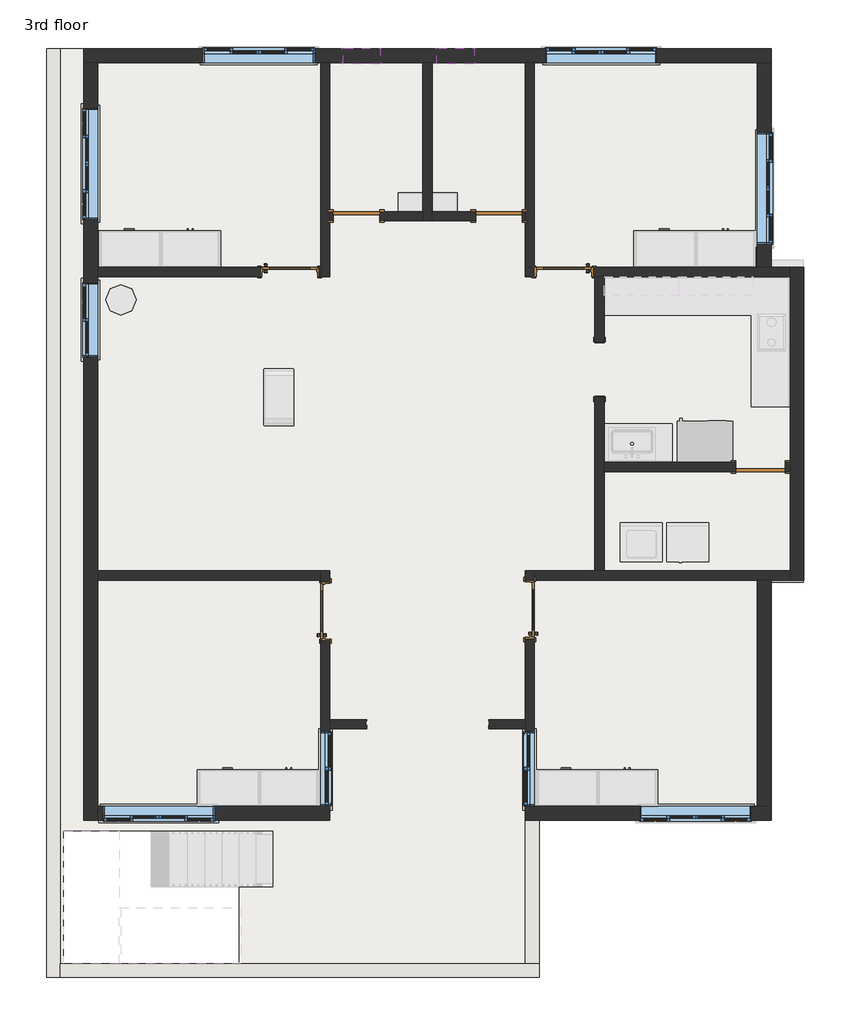
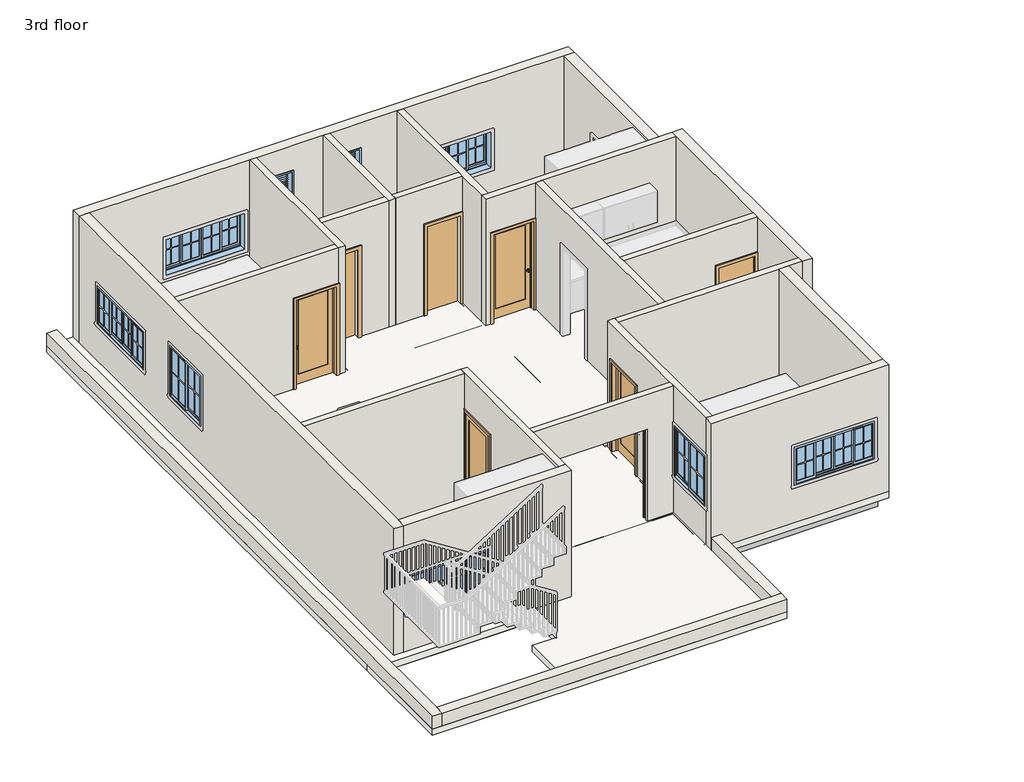
# One storey, part 1 of 4: 24 walls, 11 windows, 7 beams, 7 doors, 1 slab.
# Revit data of these elements (continued)
# Element 45 (IfcWindow, "Window-Sliding-Four : 72\" x 36\"") (continued)
#   Interior Wall Closure = 0' - 2 3/4"
#   Frame Extension = 0' - 0 1/4"
#   Exterior Wall Closure = 0' - 1 1/4"
#   Interior Trim Visibility = yes
#   Indicator Visibility = yes
#   Exterior Trim Visibility = yes
#   Phase Created = New Construction
#   Materials on its faces: "Wood - Stained", "Glass", "Clad - White"
# Element 46 (IfcWindow, "Window-Sliding-Four : 72\" x 36\"")
#   Mark = "40"
#   Window Inset = 0' - 0"
#   Interior Wall Closure = 0' - 2 3/4"
#   Frame Extension = 0' - 0 1/4"
#   Exterior Wall Closure = 0' - 1 1/4"
#   Interior Trim Visibility = yes
#   Indicator Visibility = yes
#   Exterior Trim Visibility = yes
#   Phase Created = New Construction
#   Materials on its faces: "Wood - Stained", "Glass", "Clad - White"
# Element 47 (IfcWindow, "Window-Sliding-Four : 72\" x 36\"")
#   Mark = "41"
#   Window Inset = 0' - 0"
#   Interior Wall Closure = 0' - 2 3/4"
#   Frame Extension = 0' - 0 1/4"
#   Exterior Wall Closure = 0' - 1 1/4"
#   Interior Trim Visibility = yes
#   Indicator Visibility = yes
#   Exterior Trim Visibility = yes
#   Phase Created = New Construction
#   Materials on its faces: "Wood - Stained", "Glass", "Clad - White"
# Element 48 (IfcWindow, "Window-Sliding-Four : 72\" x 36\"")
#   Mark = "42"
#   Window Inset = 0' - 0"
#   Interior Wall Closure = 0' - 2 3/4"
#   Frame Extension = 0' - 0 1/4"
#   Exterior Wall Closure = 0' - 1 1/4"
#   Interior Trim Visibility = yes
#   Indicator Visibility = yes
#   Exterior Trim Visibility = yes
#   Phase Created = New Construction
#   Materials on its faces: "Wood - Stained", "Glass", "Clad - White"
# Element 49 (IfcWindow, "Window-Sliding-Four : 72\" x 36\"")
#   Mark = "46"
#   Window Inset = 0' - 0"
#   Interior Wall Closure = 0' - 2 3/4"
#   Frame Extension = 0' - 0 1/4"
#   Exterior Wall Closure = 0' - 1 1/4"
#   Interior Trim Visibility = yes
#   Indicator Visibility = yes
#   Exterior Trim Visibility = yes
#   Phase Created = New Construction
#   Materials on its faces: "Wood - Stained", "Glass", "Clad - White"
# Element 50 (IfcWindow, "Window-Sliding-Four : 72\" x 36\"")
#   Mark = "47"
#   Window Inset = 0' - 0"
#   Interior Wall Closure = 0' - 2 3/4"
#   Frame Extension = 0' - 0 1/4"
#   Exterior Wall Closure = 0' - 1 1/4"
#   Interior Trim Visibility = yes
#   Indicator Visibility = yes
#   Exterior Trim Visibility = yes
#   Phase Created = New Construction
#   Materials on its faces: "Wood - Stained", "Glass", "Clad - White"
# Materials
#   "Concrete, Cast-in-Place gray": class "Concrete", colour RGB 192 192 192, transparency 0, Description = "Cast-in-place concrete", Cost = 0
#   "Cherry": class "Wood", colour RGB 226 177 128, transparency 0, Description = "Prunus Serotina", Cost = 0
#   "Aluminum": class "Metal", colour RGB 247 247 247, transparency 0, Description = "Aluminum 6061", Cost = 0
#   "Door - Panel": class "Wood", colour RGB 210 159 95, transparency 0, Cost = 0
#   "Door - Frame": colour RGB 118 70 51, transparency 0, Cost = 0
#   "Birch": class "Wood", colour RGB 224 178 126, transparency 0, Description = "Betula Alleghaniensis", Cost = 0
#   "Wood - Stained": class "Wood", colour RGB 224 178 126, transparency 0, Cost = 0
#   "Glass": class "Glass", colour RGB 0 128 192, transparency 0.75, Description = "Soda Lime Glass", Cost = 0
#   "Clad - White": class "Wood", colour RGB 242 242 238, transparency 0, Cost = 0
#   "Default Floor": colour RGB 128 128 128, transparency 0, Cost = 0
#   "Default Wall": colour RGB 128 128 128, transparency 0, Cost = 0
